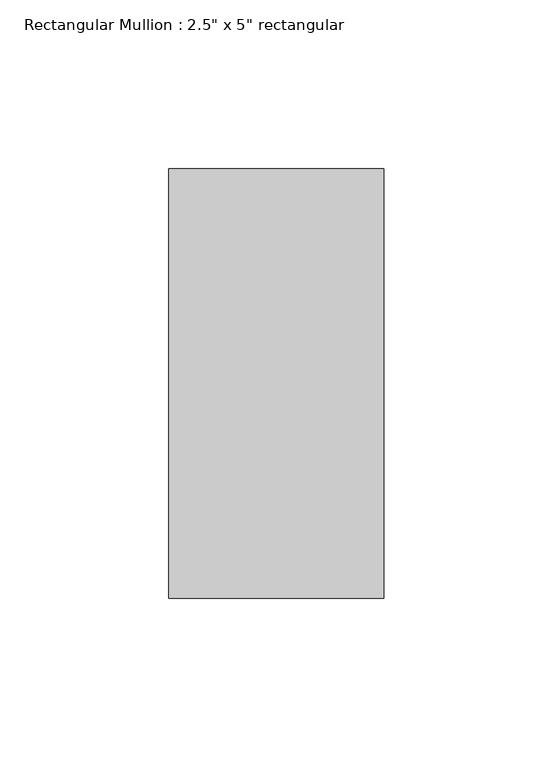
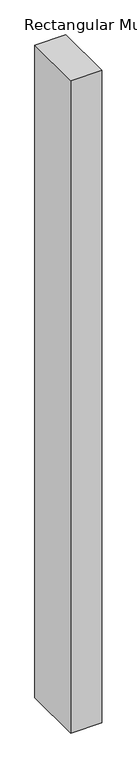
"""IFC4 building model written with IfcOpenShell, lengths in millimetres: member geometry."""

from ifc_helpers import new_model, si_unit, frame, origin, place, context, project, spatial, polyline, outline, extrude, source, transform, mapped, element, save


def member_53538a1b(model_context):
    return source(origin(), model_context, "Body", "SweptSolid", [
        extrude(outline(polyline([(0.0, 63.5), (0.0, -63.5), (-63.5, -63.5), (-63.5, 63.5), (0.0, 63.5)])), frame((0.0, 0.0, -1415.2614699), z_axis=(0.0, 0.0, 1.0), x_axis=(1.0, 0.0, 0.0)), (0.0, 0.0, 1.0), 1415.2614699),
    ])


if __name__ == "__main__":
    model = new_model("IFC4")
    model_context = context("Model", 3, world=origin())
    ifc_project = project(units=[si_unit("LENGTHUNIT", "METRE", prefix="MILLI")], contexts=[model_context])
    site = spatial("IfcSite", under=ifc_project)
    building = spatial("IfcBuilding", under=site)
    placement = place(None, origin())
    member_shape = member_53538a1b(model_context)
    element("IfcMember", 1, ObjectType="Rectangular Mullion : 2.5\" x 5\" rectangular", at=placement, inside=building, context=model_context, shape_type="MappedRepresentation", body=[
        mapped(member_shape, transform((0.0, 0.0, 0.0), x_axis=(1.0, 0.0, 0.0), y_axis=(0.0, 1.0, 0.0), z_axis=(0.0, 0.0, 1.0))),
    ])
    save(model, "model.ifc")

# Revit data of these elements
# Type "Rectangular Mullion : 2.5\" x 5\" rectangular"
#   built-in parameter 1007304 = 0.416667 (stored number, unit not read)
#   built-in parameter 1007301 = 0.104167 (stored number, unit not read)
#   built-in parameter 1007300 = 0.104167 (stored number, unit not read)
# Element 1 (IfcMember, "Rectangular Mullion : 2.5\" x 5\" rectangular")
#   Materials on its faces: "Aluminum"
# Materials
#   "Aluminum": class "Metal", colour RGB 247 247 247, transparency 0, Description = "Aluminum 6061", Cost = 0
